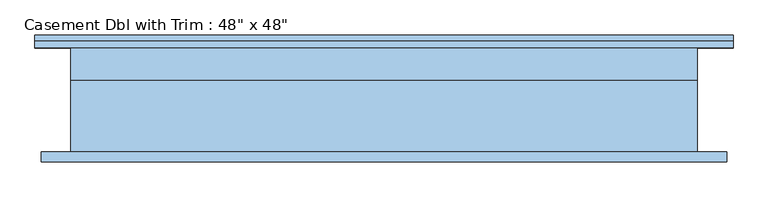
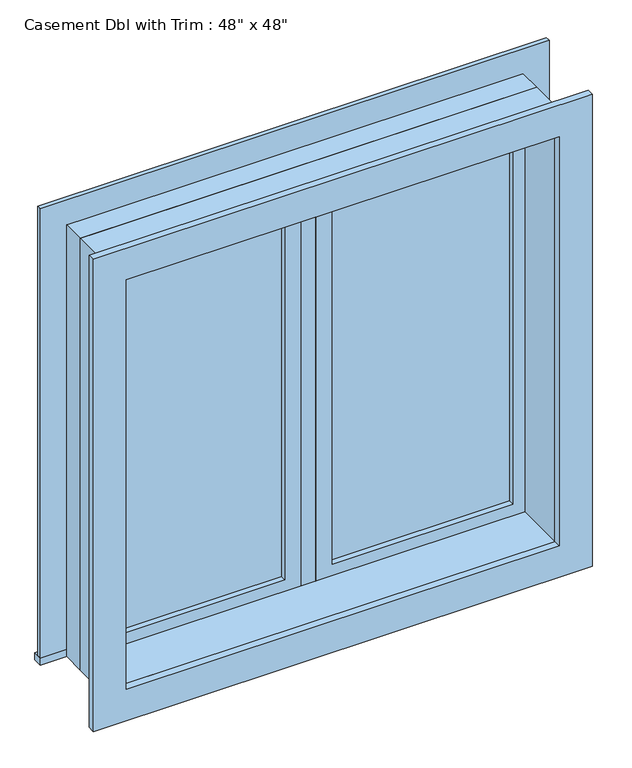
"""IFC4 building model written with IfcOpenShell, lengths in millimetres: window geometry."""

from ifc_helpers import new_model, si_unit, frame, origin, place, context, project, spatial, polyline, outline, extrude, source, transform, mapped, element, save


def window_0862ab64(model_context):
    return source(origin(), model_context, "Body", "SweptSolid", [
        extrude(outline(polyline([(63.5, 85.725), (546.1, 85.725), (546.1, 73.025), (63.5, 73.025), (63.5, 85.725)])), frame((0.0, 0.0, 977.9), z_axis=(0.0, 0.0, 1.0), x_axis=(1.0, 0.0, 0.0)), (0.0, 0.0, 1.0), 1092.2),
        extrude(outline(polyline([(2114.55, 19.05), (933.45, 19.05), (933.45, 590.55), (2114.55, 590.55), (2114.55, 19.05)]), holes=[polyline([(2070.1, 63.5), (2070.1, 546.1), (977.9, 546.1), (977.9, 63.5), (2070.1, 63.5)])]), frame((0.0, 57.15, 0.0), z_axis=(0.0, 1.0, 0.0), x_axis=(0.0, 0.0, 1.0)), (0.0, 0.0, 1.0), 44.45),
        extrude(outline(polyline([(19.05, 57.15), (-19.05, 57.15), (-19.05, 120.65), (19.05, 120.65), (19.05, 57.15)])), frame((0.0, 0.0, 933.45), z_axis=(0.0, 0.0, 1.0), x_axis=(1.0, 0.0, 0.0)), (0.0, 0.0, 1.0), 1181.1),
        extrude(outline(polyline([(-679.45, 146.05), (679.45, 146.05), (679.45, 120.65), (-679.45, 120.65), (-679.45, 146.05)])), frame((0.0, 0.0, 914.4), z_axis=(0.0, 0.0, 1.0), x_axis=(1.0, 0.0, 0.0)), (0.0, 0.0, 1.0), 19.05),
        extrude(outline(polyline([(2114.55, -590.55), (2114.55, 590.55), (933.45, 590.55), (933.45, 679.45), (2203.45, 679.45), (2203.45, -679.45), (933.45, -679.45), (933.45, -590.55), (2114.55, -590.55)])), frame((0.0, 120.65, 0.0), z_axis=(0.0, 1.0, 0.0), x_axis=(0.0, 0.0, 1.0)), (0.0, 0.0, 1.0), 12.7),
        extrude(outline(polyline([(2190.75, 666.75), (2190.75, -666.75), (857.25, -666.75), (857.25, 666.75), (2190.75, 666.75)]), holes=[polyline([(2101.85, 577.85), (946.15, 577.85), (946.15, -577.85), (2101.85, -577.85), (2101.85, 577.85)])]), frame((0.0, -101.6, 0.0), z_axis=(0.0, 1.0, 0.0), x_axis=(0.0, 0.0, 1.0)), (0.0, 0.0, 1.0), 19.05),
        extrude(outline(polyline([(-63.5, 73.025), (-546.1, 73.025), (-546.1, 85.725), (-63.5, 85.725), (-63.5, 73.025)])), frame((0.0, 0.0, 977.9), z_axis=(0.0, 0.0, 1.0), x_axis=(1.0, 0.0, 0.0)), (0.0, 0.0, 1.0), 1092.2),
        extrude(outline(polyline([(2114.55, -590.55), (933.45, -590.55), (933.45, -19.05), (2114.55, -19.05), (2114.55, -590.55)]), holes=[polyline([(2070.1, -546.1), (2070.1, -63.5), (977.9, -63.5), (977.9, -546.1), (2070.1, -546.1)])]), frame((0.0, 57.15, 0.0), z_axis=(0.0, 1.0, 0.0), x_axis=(0.0, 0.0, 1.0)), (0.0, 0.0, 1.0), 44.45),
        extrude(outline(polyline([(2133.6, -609.6), (914.4, -609.6), (914.4, 609.6), (2133.6, 609.6), (2133.6, -609.6)]), holes=[polyline([(2101.85, -577.85), (2101.85, 577.85), (946.15, 577.85), (946.15, -577.85), (2101.85, -577.85)])]), frame((0.0, -82.55, 0.0), z_axis=(0.0, 1.0, 0.0), x_axis=(0.0, 0.0, 1.0)), (0.0, 0.0, 1.0), 139.7),
        extrude(outline(polyline([(2133.6, 609.6), (2133.6, -609.6), (914.4, -609.6), (914.4, 609.6), (2133.6, 609.6)]), holes=[polyline([(2114.55, 590.55), (933.45, 590.55), (933.45, -590.55), (2114.55, -590.55), (2114.55, 590.55)])]), frame((0.0, 57.15, 0.0), z_axis=(0.0, 1.0, 0.0), x_axis=(0.0, 0.0, 1.0)), (0.0, 0.0, 1.0), 63.5),
    ])


if __name__ == "__main__":
    model = new_model("IFC4")
    model_context = context("Model", 3, world=origin())
    ifc_project = project(units=[si_unit("LENGTHUNIT", "METRE", prefix="MILLI")], contexts=[model_context])
    site = spatial("IfcSite", under=ifc_project)
    building = spatial("IfcBuilding", under=site)
    placement = place(None, origin())
    window_shape = window_0862ab64(model_context)
    element("IfcWindow", 1, ObjectType="Casement Dbl with Trim : 48\" x 48\"", at=placement, inside=building, context=model_context, shape_type="MappedRepresentation", body=[
        mapped(window_shape, transform((0.0, 0.0, 0.0), x_axis=(1.0, 0.0, 0.0), y_axis=(0.0, 1.0, 0.0), z_axis=(0.0, 0.0, 1.0))),
    ])
    save(model, "model.ifc")

# Revit data of these elements
# Type "Casement Dbl with Trim : 48\" x 48\""
#   Type Mark = "19"
#   Construction Type Id = "GSP4R"
#   Assembly Code = "B2020100"
#   Analytic Construction = "1/8 in Pilkington single glazing"
#   Visual Light Transmittance = 0.9
#   Solar Heat Gain Coefficient = 0.78
#   Heat Transfer Coefficient (U) = 0.6496 BTU/(h·ft²·°F)
#   Height = 4' - 0"
#   Default Sill Height = 3' - 0"
#   Trim Projection - Ext. = 0' - 0 1/2"
#   Trim Projection - Int. = 0' - 0 3/4"
#   Trim Width - Exterior = 0' - 3 1/2"
#   Trim Width - Interior = 0' - 3 1/2"
#   Width = 4' - 0"
#   Window Inset = 0' - 0 3/4"
#   Define Thermal Properties by = 1
#   Glass Pane Material = Glass
#   Sash Material = Sash
#   Trim Exterior Material = Trim
#   Trim Interior Material = Trim
#   Wall Closure = (empty or 0)
# Element 1 (IfcWindow, "Casement Dbl with Trim : 48\" x 48\"")
#   Materials on its faces: "Sash", "Trim", "Glass"
# Materials
#   "Glass": class "Glass", colour RGB 0 128 192, transparency 0.75, Description = "Soda Lime Glass", Cost = 0
#   "Sash": class "Wood", colour RGB 224 178 126, transparency 0
#   "Trim": class "Wood", colour RGB 224 178 126, transparency 0
